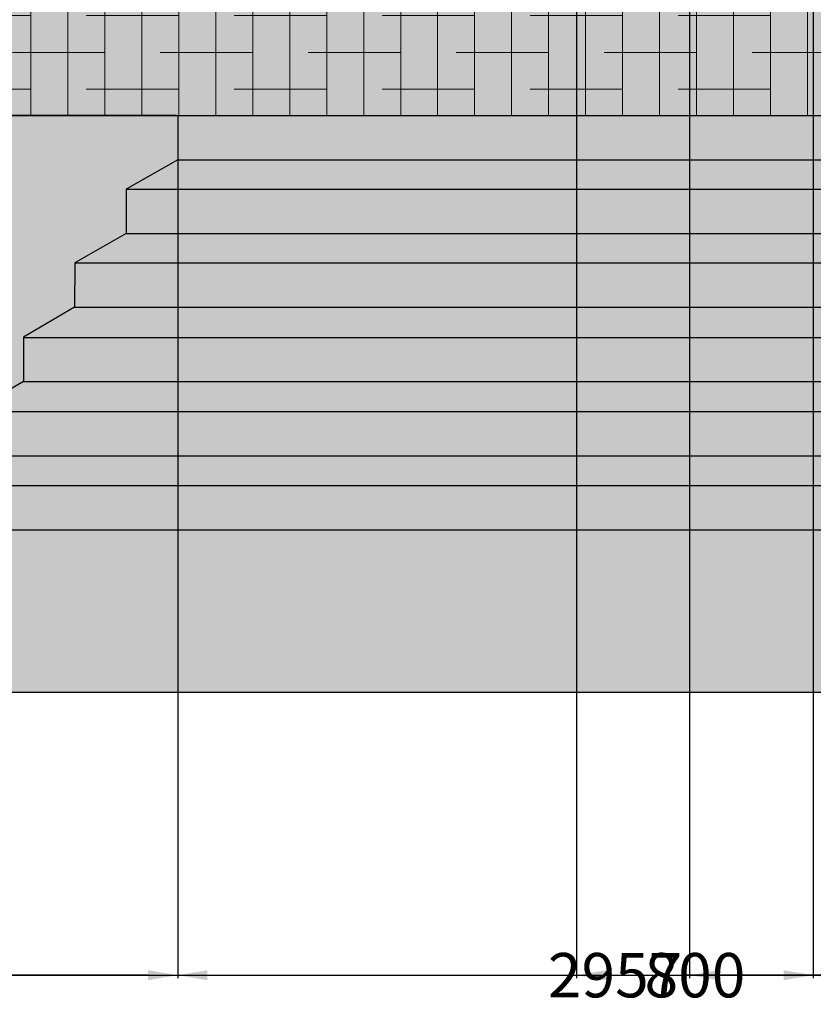
# Model space of a CAD drawing. Units: millimetres. Extents: x 11032 to 26788, y 3406 to 24505.
# Tile 2 of 78: x 14462 to 17145, y 3406 to 6736. Entities that reach past the tile are written whole.
import ezdxf

# ---------------------------------------------------------------- set-up
doc = ezdxf.new("R2010")
doc.units = ezdxf.units.MM
doc.header["$MEASUREMENT"] = 0
for name, color, linetype, lineweight in [('A-ANNO-DIMS', 2, 'Continuous', 18), ('A-FLOR-STRS', 7, 'Continuous', 25), ('A-FLOR-STRS-PATT', 8, 'Continuous', 13), ('A-WALL-PLIN', 7, 'Continuous', 30), ('A-WALL-PLIN-PATT', 253, 'Continuous', 13), ('L-PLNT-PATT', 92, 'Continuous', 13)]:
    doc.layers.add(name, color=color, linetype=linetype, lineweight=lineweight)
doc.styles.get("Standard").update_dxf_attribs({"font": 'arial.ttf'})
doc.dimstyles.get("Standard").update_dxf_attribs({"dimtxt": 150, "dimasz": 100, "dimexe": 10, "dimexo": 5, "dimgap": 5, "dimtad": 0, "dimtih": 1, "dimtoh": 1, "dimdec": 0, "dimzin": 0, "dimdsep": 46, "dimtxsty": 'Standard', "dimcen": 0.09, "dimadec": 0, "dimazin": 0, "dimtfac": 1, "dimtdec": 0, "dimtofl": 0, "dimtmove": 0, "dimatfit": 3, "dimfxl": 1, "dimtolj": 1, "dimtzin": 0, "dimarcsym": 0})

# ---------------------------------------------------------------- blocks, each defined once
blk = doc.blocks.new('*D36')
at = {"layer": 'A-ANNO-DIMS', "color": 0, "lineweight": -2, "transparency": 16777216}
for p, q in [((12301.3, 17115.9), (12301.3, 24416.9)), ((12401.3, 24406.9), (18569.2, 24406.9)), ((25297.4, 24406.9), (19129.5, 24406.9)), ((25397.4, 4466.4), (25397.4, 24416.9))]:
    blk.add_line(p, q, dxfattribs=at)
at = {"layer": 'A-ANNO-DIMS', "color": 0, "transparency": 16777216}
for points in [[(12401.3, 24423.5), (12401.3, 24390.2), (12301.3, 24406.9)], [(25297.4, 24423.5), (25297.4, 24390.2), (25397.4, 24406.9)]]:
    blk.add_solid(points, dxfattribs=at)
at = {"layer": 'Defpoints', "color": 0, "transparency": 16777216}
for p in [(25397.4, 24406.9), (12301.3, 17110.9), (25397.4, 4461.4)]:
    blk.add_point(p, dxfattribs=at)
at = {"layer": 'A-ANNO-DIMS', "color": 0, "transparency": 16777216, "insert": (18849.3, 24406.9), "char_height": 150, "attachment_point": 5}
blk.add_mtext('\\A1;13096', dxfattribs=at)
blk = doc.blocks.new('*D37')
at = {"layer": 'A-ANNO-DIMS', "color": 0, "lineweight": -2, "transparency": 16777216}
for p, q in [((18087.7, 23450.4), (11334.8, 23450.4)), ((11344.8, 23350.4), (11344.8, 14037.5)), ((11344.8, 4561.4), (11344.8, 13874.3)), ((12927.7, 4461.4), (11334.8, 4461.4))]:
    blk.add_line(p, q, dxfattribs=at)
at = {"layer": 'A-ANNO-DIMS', "color": 0, "transparency": 16777216}
for points in [[(11328.1, 23350.4), (11361.4, 23350.4), (11344.8, 23450.4)], [(11328.1, 4561.4), (11361.4, 4561.4), (11344.8, 4461.4)]]:
    blk.add_solid(points, dxfattribs=at)
at = {"layer": 'Defpoints', "color": 0, "transparency": 16777216}
for p in [(11344.8, 23450.4), (18092.7, 23450.4), (12932.7, 4461.4)]:
    blk.add_point(p, dxfattribs=at)
at = {"layer": 'A-ANNO-DIMS', "color": 0, "transparency": 16777216, "insert": (11344.8, 13955.9), "char_height": 150, "attachment_point": 5}
blk.add_mtext('\\A1;18989', dxfattribs=at)
blk = doc.blocks.new('*D48')
at = {"layer": 'A-ANNO-DIMS', "color": 0, "lineweight": -2, "transparency": 16777216}
for p, q in [((14996.4, 6406.4), (14996.4, 3494.9)), ((12932.7, 4456.4), (12932.7, 3494.9)), ((13032.7, 3504.9), (13646.9, 3504.9)), ((14896.4, 3504.9), (14282.2, 3504.9))]:
    blk.add_line(p, q, dxfattribs=at)
at = {"layer": 'A-ANNO-DIMS', "color": 0, "transparency": 16777216}
for points in [[(13032.7, 3521.6), (13032.7, 3488.2), (12932.7, 3504.9)], [(14896.4, 3521.6), (14896.4, 3488.2), (14996.4, 3504.9)]]:
    blk.add_solid(points, dxfattribs=at)
at = {"layer": 'Defpoints', "color": 0, "transparency": 16777216}
for p in [(14996.4, 6411.4), (12932.7, 4461.4), (14996.4, 3504.9)]:
    blk.add_point(p, dxfattribs=at)
at = {"layer": 'A-ANNO-DIMS', "color": 0, "transparency": 16777216, "insert": (13964.5, 3504.9), "char_height": 150, "attachment_point": 5}
blk.add_mtext('\\A1;2063.7', dxfattribs=at)
blk = doc.blocks.new('*D49')
at = {"layer": 'A-ANNO-DIMS', "color": 0, "lineweight": -2, "transparency": 16777216}
for p, q in [((17953.5, 10206.4), (17953.5, 3494.9)), ((14996.4, 6406.4), (14996.4, 3494.9)), ((15096.4, 3504.9), (16244.7, 3504.9)), ((17853.5, 3504.9), (16705.2, 3504.9))]:
    blk.add_line(p, q, dxfattribs=at)
at = {"layer": 'A-ANNO-DIMS', "color": 0, "transparency": 16777216}
for points in [[(15096.4, 3521.6), (15096.4, 3488.2), (14996.4, 3504.9)], [(17853.5, 3521.6), (17853.5, 3488.2), (17953.5, 3504.9)]]:
    blk.add_solid(points, dxfattribs=at)
at = {"layer": 'Defpoints', "color": 0, "transparency": 16777216}
for p in [(17953.5, 10211.4), (14996.4, 6411.4), (17953.5, 3504.9)]:
    blk.add_point(p, dxfattribs=at)
at = {"layer": 'A-ANNO-DIMS', "color": 0, "transparency": 16777216, "insert": (16474.9, 3504.9), "char_height": 150, "attachment_point": 5}
blk.add_mtext('\\A1;2957', dxfattribs=at)
blk = doc.blocks.new('*D55')
at = {"layer": 'A-ANNO-DIMS', "color": 0, "lineweight": -2, "transparency": 16777216}
for p, q in [((14128.4, 5006.1), (14128.4, 3494.9)), ((21761, 5006.1), (21761, 3494.9)), ((14228.4, 3504.9), (17716.3, 3504.9)), ((21661, 3504.9), (18173.1, 3504.9))]:
    blk.add_line(p, q, dxfattribs=at)
at = {"layer": 'A-ANNO-DIMS', "color": 0, "transparency": 16777216}
for points in [[(14228.4, 3521.6), (14228.4, 3488.2), (14128.4, 3504.9)], [(21661, 3521.6), (21661, 3488.2), (21761, 3504.9)]]:
    blk.add_solid(points, dxfattribs=at)
at = {"layer": 'Defpoints', "color": 0, "transparency": 16777216}
for p in [(14128.4, 5011.1), (21761, 5011.1), (21761, 3504.9)]:
    blk.add_point(p, dxfattribs=at)
at = {"layer": 'A-ANNO-DIMS', "color": 0, "transparency": 16777216, "insert": (17944.7, 3504.9), "char_height": 150, "attachment_point": 5}
blk.add_mtext('\\A1;7633', dxfattribs=at)
blk = doc.blocks.new('*D56')
at = {"layer": 'A-ANNO-DIMS', "color": 0, "lineweight": -2, "transparency": 16777216}
for p, q in [((14991.4, 6411.4), (11334.8, 6411.4)), ((11344.8, 6311.4), (11344.8, 5792.9)), ((11344.8, 5111.1), (11344.8, 5629.6)), ((14123.4, 5011.1), (11334.8, 5011.1))]:
    blk.add_line(p, q, dxfattribs=at)
at = {"layer": 'A-ANNO-DIMS', "color": 0, "transparency": 16777216}
for points in [[(11328.1, 6311.4), (11361.4, 6311.4), (11344.8, 6411.4)], [(11328.1, 5111.1), (11361.4, 5111.1), (11344.8, 5011.1)]]:
    blk.add_solid(points, dxfattribs=at)
at = {"layer": 'Defpoints', "color": 0, "transparency": 16777216}
for p in [(11344.8, 6411.4), (14996.4, 6411.4), (14128.4, 5011.1)]:
    blk.add_point(p, dxfattribs=at)
at = {"layer": 'A-ANNO-DIMS', "color": 0, "transparency": 16777216, "insert": (11344.8, 5711.2), "char_height": 150, "attachment_point": 5}
blk.add_mtext('\\A1;1400.3', dxfattribs=at)
blk = doc.blocks.new('*D61')
at = {"layer": 'A-ANNO-DIMS', "color": 0, "lineweight": -2, "transparency": 16777216}
for p, q in [((17144.7, 7306.4), (17144.7, 3494.9)), ((16344.7, 7256.4), (16344.7, 3494.9)), ((16444.7, 3504.9), (16574.2, 3504.9)), ((17044.7, 3504.9), (16915.3, 3504.9))]:
    blk.add_line(p, q, dxfattribs=at)
at = {"layer": 'A-ANNO-DIMS', "color": 0, "transparency": 16777216}
for points in [[(16444.7, 3521.6), (16444.7, 3488.2), (16344.7, 3504.9)], [(17044.7, 3521.6), (17044.7, 3488.2), (17144.7, 3504.9)]]:
    blk.add_solid(points, dxfattribs=at)
at = {"layer": 'Defpoints', "color": 0, "transparency": 16777216}
for p in [(17144.7, 7311.4), (16344.7, 7261.4), (17144.7, 3504.9)]:
    blk.add_point(p, dxfattribs=at)
at = {"layer": 'A-ANNO-DIMS', "color": 0, "transparency": 16777216, "insert": (16744.7, 3504.9), "char_height": 150, "attachment_point": 5}
blk.add_mtext('\\A1;800', dxfattribs=at)
blk = doc.blocks.new('*D62')
at = {"layer": 'A-ANNO-DIMS', "color": 0, "lineweight": -2, "transparency": 16777216}
for p, q in [((17144.7, 7306.4), (17144.7, 3494.9)), ((17944.7, 7256.4), (17944.7, 3494.9)), ((17244.7, 3504.9), (17374.2, 3504.9)), ((17844.7, 3504.9), (17715.3, 3504.9))]:
    blk.add_line(p, q, dxfattribs=at)
at = {"layer": 'A-ANNO-DIMS', "color": 0, "transparency": 16777216}
for points in [[(17244.7, 3521.6), (17244.7, 3488.2), (17144.7, 3504.9)], [(17844.7, 3521.6), (17844.7, 3488.2), (17944.7, 3504.9)]]:
    blk.add_solid(points, dxfattribs=at)
at = {"layer": 'Defpoints', "color": 0, "transparency": 16777216}
for p in [(17144.7, 7311.4), (17944.7, 7261.4), (17944.7, 3504.9)]:
    blk.add_point(p, dxfattribs=at)
at = {"layer": 'A-ANNO-DIMS', "color": 0, "transparency": 16777216, "insert": (17544.7, 3504.9), "char_height": 150, "attachment_point": 5}
blk.add_mtext('\\A1;800', dxfattribs=at)
blk = doc.blocks.new('*D66')
at = {"layer": 'A-ANNO-DIMS', "color": 0, "lineweight": -2, "transparency": 16777216}
for p, q in [((16725.9, 10296), (16725.9, 3494.9)), ((19150.9, 10296), (19150.9, 3494.9)), ((16825.9, 3504.9), (17707.6, 3504.9)), ((19050.9, 3504.9), (18169.3, 3504.9))]:
    blk.add_line(p, q, dxfattribs=at)
at = {"layer": 'A-ANNO-DIMS', "color": 0, "transparency": 16777216}
for points in [[(16825.9, 3521.6), (16825.9, 3488.2), (16725.9, 3504.9)], [(19050.9, 3521.6), (19050.9, 3488.2), (19150.9, 3504.9)]]:
    blk.add_solid(points, dxfattribs=at)
at = {"layer": 'Defpoints', "color": 0, "transparency": 16777216}
for p in [(16725.9, 10301), (19150.9, 10301), (19150.9, 3504.9)]:
    blk.add_point(p, dxfattribs=at)
at = {"layer": 'A-ANNO-DIMS', "color": 0, "transparency": 16777216, "insert": (17938.4, 3504.9), "char_height": 150, "attachment_point": 5}
blk.add_mtext('\\A1;2425', dxfattribs=at)

msp = doc.modelspace()

# ---------------------------------------------------------------- hatches: boundary and pattern name
at = {"layer": 'A-FLOR-STRS-PATT'}
h = msp.add_hatch(color=256, dxfattribs=at)
h.set_gradient(color1=(99, 100, 102), color2=(199, 200, 202), name='INVCYLINDER')
h.paths.add_polyline_path([(14996.399, 6411.399), (14996.399, 6261.399), (20893.008, 6261.399), (20893.008, 6411.399)])
h.paths.add_polyline_path([(21067.183, 6012.807), (21067.019, 6162.807), (14822.389, 6162.807), (14822.224, 6012.807)])
h.paths.add_polyline_path([(21241.977, 5763.336), (21240.69, 5913.331), (14648.718, 5913.331), (14647.43, 5763.336)])
h.paths.add_polyline_path([(14474.774, 5661.399), (14474.964, 5512.395), (21414.443, 5512.395), (21414.634, 5661.399)])
h.paths.add_polyline_path([(14302.433, 5411.236), (14301.435, 5261.24), (21587.972, 5261.24), (21586.974, 5411.236)])
h.paths.add_polyline_path([(14128.313, 5161.097), (14128.428, 5011.097), (21760.979, 5011.097), (21761.094, 5161.097)])
at = {"layer": 'A-WALL-PLIN-PATT'}
h = msp.add_hatch(color=256, dxfattribs=at)
h.set_gradient(color1=(99, 100, 102), color2=(199, 200, 202), name='CYLINDER')
edge = h.paths.add_edge_path()
edge.add_arc((17944.704, 7261.399), 2950, 180, 181.942602)
edge.add_line((14996.399, 7161.399), (12932.665, 7161.399))
edge.add_line((12932.665, 7161.399), (12932.665, 6411.399))
edge.add_line((12932.665, 6411.399), (25397.404, 6411.399))
edge.add_line((25397.404, 6411.399), (25397.404, 7161.399))
edge.add_line((25397.404, 7161.399), (22955.171, 7161.399))
edge.add_spline(control_points=[(22955.171, 7161.399), (22875.95, 7159.113), (22796.729, 7156.828), (22718.347, 7161.399)], knot_values=[0, 0, 0, 0, 236.62389499, 236.62389499, 236.62389499, 236.62389499], degree=3, periodic=0)
edge.add_spline(control_points=[(22718.347, 7161.399), (22709.27, 7161.929), (22517.84, 7175.049), (22332.009, 7233.921), (22155.123, 7291.176)], knot_values=[236.62389499, 236.62389499, 236.62389499, 236.62389499, 264.02785008, 815.24414583, 815.24414583, 815.24414583, 815.24414583], degree=3, periodic=0)
edge.add_line((22155.123, 7291.176), (22155.123, 7161.399))
edge.add_line((22155.123, 7161.399), (20893.008, 7161.399))
edge.add_arc((17944.704, 7261.399), 2950, 358.057398, 360)
edge.add_line((20894.704, 7261.399), (14994.704, 7261.399))
h.paths.add_polyline_path([(14996.399, 6261.399), (14822.389, 6162.807), (21067.019, 6162.807), (20893.008, 6261.399)])
h.paths.add_polyline_path([(14822.224, 6012.807), (14648.718, 5913.331), (21240.69, 5913.331), (21067.183, 6012.807)])
h.paths.add_polyline_path([(21414.634, 5661.399), (21414.635, 5662.395), (21241.977, 5763.336), (14647.43, 5763.336), (14474.772, 5662.395), (14474.774, 5661.399)])
h.paths.add_polyline_path([(14474.964, 5512.395), (14302.433, 5411.236), (21586.974, 5411.236), (21414.443, 5512.395)])
h.paths.add_polyline_path([(14301.435, 5261.24), (14128.313, 5161.097), (21761.094, 5161.097), (21587.972, 5261.24)])
h.paths.add_polyline_path([(22722.526, 4461.399), (21760.979, 5011.097), (14128.428, 5011.097), (13166.882, 4461.399)])
h = msp.add_hatch(dxfattribs=at)
h.set_pattern_fill('ANSI38', color=256, scale=1000, angle=45, style=0)
edge = h.paths.add_edge_path()
edge.add_line((25397.404, 6411.399), (25397.404, 7161.399))
edge.add_line((25397.404, 7161.399), (22955.171, 7161.399))
edge.add_spline(control_points=[(22955.171, 7161.399), (22875.95, 7159.113), (22796.729, 7156.828), (22718.347, 7161.399)], knot_values=[0, 0, 0, 0, 236.62389499, 236.62389499, 236.62389499, 236.62389499], degree=3, periodic=0)
edge.add_spline(control_points=[(22718.347, 7161.399), (22709.27, 7161.929), (22517.84, 7175.049), (22332.009, 7233.921), (22155.123, 7291.176)], knot_values=[236.62389499, 236.62389499, 236.62389499, 236.62389499, 264.02785008, 815.24414583, 815.24414583, 815.24414583, 815.24414583], degree=3, periodic=0)
edge.add_line((22155.123, 7291.176), (22155.123, 7161.399))
edge.add_line((22155.123, 7161.399), (20893.008, 7161.399))
edge.add_arc((17944.704, 7261.399), 2950, 358.057398, 360)
edge.add_line((20894.704, 7261.399), (14994.704, 7261.399))
edge.add_arc((17944.704, 7261.399), 2950, 180, 181.942602)
edge.add_line((14996.399, 7161.399), (12932.665, 7161.399))
edge.add_line((12932.665, 7161.399), (12932.665, 6411.399))
edge.add_line((12932.665, 6411.399), (25397.404, 6411.399))
at = {"layer": 'L-PLNT-PATT'}
h = msp.add_hatch(color=256, dxfattribs=at)
h.set_gradient(color1=(19, 155, 72), color2=(0, 127, 0), name='HEMISPHERICAL')
h.paths.add_polyline_path([(12932.665, 4461.399), (13166.882, 4461.399), (14128.428, 5011.097), (14128.313, 5161.097), (14301.435, 5261.24), (14302.433, 5411.236), (14474.964, 5512.395), (14474.772, 5662.395), (14647.43, 5763.336), (14648.718, 5913.331), (14822.224, 6012.807), (14822.389, 6162.807), (14996.399, 6261.399), (14996.399, 6411.399), (12932.665, 6411.399)])

# ---------------------------------------------------------------- linework, layer by layer
at = {"layer": 'A-FLOR-STRS'}
for p, q in [((14996.399, 6411.399), (14996.399, 6261.399)), ((14996.399, 6261.399), (14822.389, 6162.807)), ((14996.399, 6261.399), (20893.008, 6261.399)), ((14822.389, 6162.807), (14822.224, 6012.807)), ((14822.389, 6162.807), (21067.019, 6162.807)), ((14822.224, 6012.807), (14648.718, 5913.331)), ((14822.224, 6012.807), (21067.183, 6012.807)), ((14648.718, 5913.331), (14647.43, 5763.336)), ((14648.718, 5913.331), (21240.69, 5913.331)), ((14647.43, 5763.336), (14474.772, 5662.395)), ((14647.43, 5763.336), (21241.977, 5763.336)), ((14474.772, 5662.395), (14474.964, 5512.395)), ((14474.774, 5661.399), (21414.634, 5661.399)), ((14474.964, 5512.395), (14302.433, 5411.236)), ((14474.964, 5512.395), (21414.443, 5512.395)), ((14302.433, 5411.236), (21586.974, 5411.236)), ((14301.435, 5261.24), (21587.972, 5261.24)), ((14128.313, 5161.097), (21761.094, 5161.097)), ((14128.428, 5011.097), (21760.979, 5011.097))]:
    msp.add_line(p, q, dxfattribs=at)
at = {"layer": 'A-WALL-PLIN'}
for p, q in [((12932.665, 6411.399), (25397.404, 6411.399)), ((12932.665, 4461.399), (25397.404, 4461.399))]:
    msp.add_line(p, q, dxfattribs=at)

# ---------------------------------------------------------------- dimensions: what is measured, and where the dimension line sits
at = {"layer": 'A-ANNO-DIMS'}
for base, p1, p2, override, picture, middle in [((25397.404, 24406.858), (12301.265, 17110.885), (25397.404, 4461.399), {"dimdec": 0, "dimlfac": 1, "dimrnd": 0, "dimzin": 0, "dimdsep": 46, "dimlunit": 2}, '*D36', (18849.334, 24406.858)), ((19150.949, 3504.899), (16725.949, 10301.016), (19150.949, 10301.016), {"dimdec": 0, "dimlfac": 1, "dimrnd": 0, "dimzin": 0, "dimdsep": 46, "dimlunit": 2}, '*D66', (17938.449, 3504.899)), ((17953.455, 3504.899), (14996.399, 6411.399), (17953.455, 10211.41), {"dimdec": 0, "dimlfac": 1, "dimrnd": 0, "dimzin": 0, "dimdsep": 46, "dimlunit": 2}, '*D49', (16474.927, 3504.899)), ((17144.704, 3504.899), (16344.704, 7261.399), (17144.704, 7311.399), {"dimdec": 0, "dimlfac": 1, "dimrnd": 0, "dimzin": 0, "dimdsep": 46, "dimlunit": 2}, '*D61', (16744.704, 3504.899)), ((17944.704, 3504.899), (17144.704, 7311.399), (17944.704, 7261.399), {"dimdec": 0, "dimlfac": 1, "dimrnd": 0, "dimzin": 0, "dimdsep": 46, "dimlunit": 2}, '*D62', (17544.704, 3504.899)), ((14996.399, 3504.899), (12932.665, 4461.399), (14996.399, 6411.399), {"dimdec": 1, "dimlfac": 1, "dimrnd": 0, "dimzin": 0, "dimdsep": 46, "dimlunit": 2}, '*D48', (13964.532, 3504.899)), ((21760.979, 3504.899), (14128.428, 5011.097), (21760.979, 5011.097), {"dimdec": 0, "dimlfac": 1, "dimrnd": 0, "dimzin": 0, "dimdsep": 46, "dimlunit": 2}, '*D55', (17944.704, 3504.899))]:
    dim = msp.add_linear_dim(base=base, p1=p1, p2=p2, dimstyle='Standard', override=override, dxfattribs=at)
    dim.commit()
    dim.dimension.update_dxf_attribs({"geometry": picture, "text_midpoint": middle})
for base, p1, p2, override, picture, middle in [((11344.765, 23450.358), (12932.665, 4461.399), (18092.739, 23450.358), {"dimdec": 0, "dimlfac": 1, "dimrnd": 0, "dimzin": 0, "dimdsep": 46, "dimlunit": 2}, '*D37', (11344.765, 13955.879)), ((11344.765, 6411.399), (14128.428, 5011.097), (14996.399, 6411.399), {"dimdec": 1, "dimlfac": 1, "dimrnd": 0, "dimzin": 0, "dimdsep": 46, "dimlunit": 2}, '*D56', (11344.765, 5711.248))]:
    dim = msp.add_linear_dim(base=base, p1=p1, p2=p2, angle=90, dimstyle='Standard', override=override, dxfattribs=at)
    dim.commit()
    dim.dimension.update_dxf_attribs({"geometry": picture, "text_midpoint": middle})

doc.saveas('drawing.dxf')
